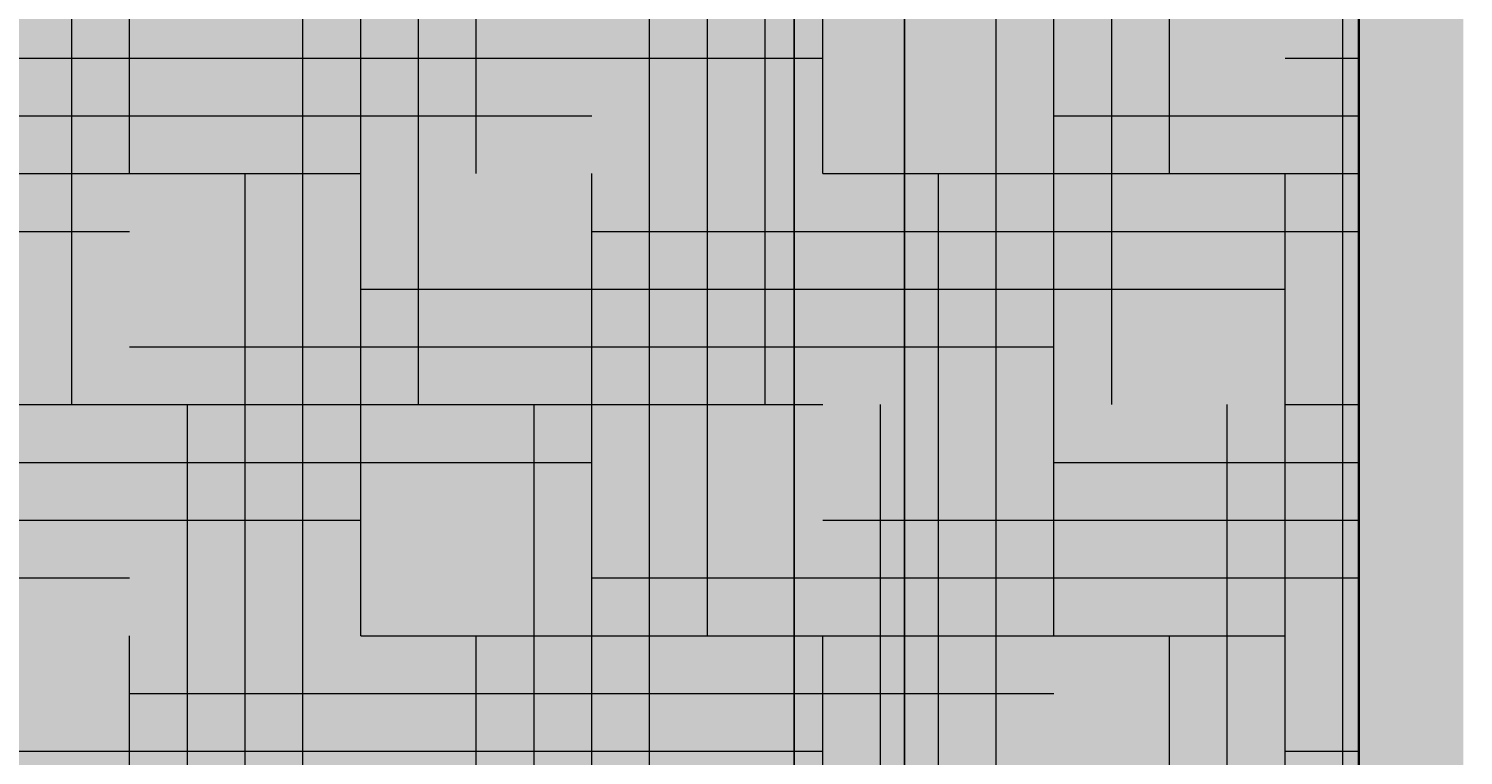
# Model space of a CAD drawing. Units: feet. Extents: x 2695 to 2912, y 795 to 1139.
# Tile 8 of 83: x 2734 to 2774, y 835 to 855. Entities that reach past the tile are written whole.
import ezdxf

# ---------------------------------------------------------------- set-up
doc = ezdxf.new("R2010")
doc.units = ezdxf.units.FT
for name, color, linetype, lineweight in [('A-ANNO-DIMS', 2, 'Continuous', 18), ('A-ELEV', 7, 'Continuous', 35), ('A-ELEV-PATT', 252, 'Continuous', 13)]:
    doc.layers.add(name, color=color, linetype=linetype, lineweight=lineweight)
doc.styles.get("Standard").update_dxf_attribs({"font": 'arial.ttf'})
doc.dimstyles.get("Standard").update_dxf_attribs({"dimtxt": 0.18, "dimasz": 0.18, "dimexe": 0.18, "dimexo": 0.0625, "dimgap": 0.09, "dimtad": 0, "dimtih": 1, "dimtoh": 1, "dimdec": 1, "dimzin": 0, "dimdsep": 46, "dimlunit": 3, "dimtxsty": 'Standard', "dimcen": 0.09, "dimadec": 0, "dimazin": 0, "dimtfac": 1, "dimtdec": 1, "dimtofl": 0, "dimtmove": 0, "dimatfit": 3, "dimfxl": 1, "dimtolj": 1, "dimtzin": 0, "dimarcsym": 0})

# ---------------------------------------------------------------- blocks, each defined once
blk = doc.blocks.new('*D3')
at = {"layer": 'A-ANNO-DIMS', "color": 0, "lineweight": -2, "transparency": 16777216}
for p, q in [((2724.189, 874.795), (2724.189, 794.976)), ((2758.151, 874.795), (2758.151, 794.976)), ((2724.369, 795.156), (2740.777, 795.156)), ((2757.971, 795.156), (2741.564, 795.156))]:
    blk.add_line(p, q, dxfattribs=at)
at = {"layer": 'A-ANNO-DIMS', "color": 0, "transparency": 16777216}
for points in [[(2724.369, 795.186), (2724.369, 795.126), (2724.189, 795.156)], [(2757.971, 795.186), (2757.971, 795.126), (2758.151, 795.156)]]:
    blk.add_solid(points, dxfattribs=at)
at = {"layer": 'Defpoints', "color": 0, "transparency": 16777216}
for p in [(2724.189, 874.857), (2758.151, 874.857), (2758.151, 795.156)]:
    blk.add_point(p, dxfattribs=at)
at = {"layer": 'A-ANNO-DIMS', "color": 0, "transparency": 16777216, "insert": (2741.17, 795.156), "char_height": 0.18, "attachment_point": 5}
blk.add_mtext('\\A1;33.96', dxfattribs=at)
blk = doc.blocks.new('*D4')
at = {"layer": 'A-ANNO-DIMS', "color": 0, "lineweight": -2, "transparency": 16777216}
for p, q in [((2758.151, 874.795), (2758.151, 794.976)), ((2773.503, 810.868), (2773.503, 794.976)), ((2758.331, 795.156), (2765.441, 795.156)), ((2773.323, 795.156), (2766.213, 795.156))]:
    blk.add_line(p, q, dxfattribs=at)
at = {"layer": 'A-ANNO-DIMS', "color": 0, "transparency": 16777216}
for points in [[(2758.331, 795.186), (2758.331, 795.126), (2758.151, 795.156)], [(2773.323, 795.186), (2773.323, 795.126), (2773.503, 795.156)]]:
    blk.add_solid(points, dxfattribs=at)
at = {"layer": 'Defpoints', "color": 0, "transparency": 16777216}
for p in [(2758.151, 874.857), (2773.503, 810.931), (2773.503, 795.156)]:
    blk.add_point(p, dxfattribs=at)
at = {"layer": 'A-ANNO-DIMS', "color": 0, "transparency": 16777216, "insert": (2765.827, 795.156), "char_height": 0.18, "attachment_point": 5}
blk.add_mtext('\\A1;15.35', dxfattribs=at)
blk = doc.blocks.new('*D13')
at = {"layer": 'A-ANNO-DIMS', "color": 0, "lineweight": -2, "transparency": 16777216}
for p, q in [((2758.214, 874.857), (2911.424, 874.857)), ((2911.244, 874.677), (2911.244, 843.076)), ((2911.244, 811.111), (2911.244, 842.712)), ((2890.699, 810.931), (2911.424, 810.931))]:
    blk.add_line(p, q, dxfattribs=at)
at = {"layer": 'A-ANNO-DIMS', "color": 0, "transparency": 16777216}
for points in [[(2911.214, 874.677), (2911.274, 874.677), (2911.244, 874.857)], [(2911.214, 811.111), (2911.274, 811.111), (2911.244, 810.931)]]:
    blk.add_solid(points, dxfattribs=at)
at = {"layer": 'Defpoints', "color": 0, "transparency": 16777216}
for p in [(2758.151, 874.857), (2911.244, 874.857), (2890.636, 810.931)]:
    blk.add_point(p, dxfattribs=at)
at = {"layer": 'A-ANNO-DIMS', "color": 0, "transparency": 16777216, "insert": (2911.244, 842.894), "char_height": 0.18, "attachment_point": 5}
blk.add_mtext('\\A1;63.93', dxfattribs=at)
blk = doc.blocks.new('*D24')
at = {"layer": 'A-ANNO-DIMS', "color": 0, "lineweight": -2, "transparency": 16777216}
for p, q in [((2730.708, 936.868), (2730.708, 794.976)), ((2755.112, 936.868), (2755.112, 794.976)), ((2730.888, 795.156), (2742.446, 795.156)), ((2754.932, 795.156), (2743.375, 795.156))]:
    blk.add_line(p, q, dxfattribs=at)
at = {"layer": 'A-ANNO-DIMS', "color": 0, "transparency": 16777216}
for points in [[(2730.888, 795.186), (2730.888, 795.126), (2730.708, 795.156)], [(2754.932, 795.186), (2754.932, 795.126), (2755.112, 795.156)]]:
    blk.add_solid(points, dxfattribs=at)
at = {"layer": 'Defpoints', "color": 0, "transparency": 16777216}
for p in [(2730.708, 936.931), (2755.112, 936.931), (2755.112, 795.156)]:
    blk.add_point(p, dxfattribs=at)
at = {"layer": 'A-ANNO-DIMS', "color": 0, "transparency": 16777216, "insert": (2742.91, 795.156), "char_height": 0.18, "attachment_point": 5}
blk.add_mtext('\\A1;24.404', dxfattribs=at)
blk = doc.blocks.new('*D25')
at = {"layer": 'A-ANNO-DIMS', "color": 0, "lineweight": -2, "transparency": 16777216}
for p, q in [((2755.112, 936.868), (2755.112, 794.976)), ((2770.636, 936.868), (2770.636, 794.976)), ((2755.292, 795.156), (2762.419, 795.156)), ((2770.456, 795.156), (2763.329, 795.156))]:
    blk.add_line(p, q, dxfattribs=at)
at = {"layer": 'A-ANNO-DIMS', "color": 0, "transparency": 16777216}
for points in [[(2755.292, 795.186), (2755.292, 795.126), (2755.112, 795.156)], [(2770.456, 795.186), (2770.456, 795.126), (2770.636, 795.156)]]:
    blk.add_solid(points, dxfattribs=at)
at = {"layer": 'Defpoints', "color": 0, "transparency": 16777216}
for p in [(2755.112, 936.931), (2770.636, 936.931), (2770.636, 795.156)]:
    blk.add_point(p, dxfattribs=at)
at = {"layer": 'A-ANNO-DIMS', "color": 0, "transparency": 16777216, "insert": (2762.874, 795.156), "char_height": 0.18, "attachment_point": 5}
blk.add_mtext('\\A1;15.524', dxfattribs=at)

msp = doc.modelspace()

# ---------------------------------------------------------------- hatches: boundary and pattern name
at = {"layer": 'A-ELEV-PATT'}
h = msp.add_hatch(color=256, dxfattribs=at)
h.set_gradient(color1=(147, 149, 152), color2=(147, 149, 152), tint=1)
h.paths.add_polyline_path([(2770.6361, 1118.4096), (2710.6361, 1118.4096), (2710.6361, 1062.9306), (2770.6361, 1062.9306)])
h.paths.add_polyline_path([(2890.6361, 1103.3378), (2770.6361, 1103.3378), (2770.6361, 1062.9306), (2890.6361, 1062.9306)])
h.paths.add_polyline_path([(2730.7081, 1048.1052), (2755.1125, 1048.1052), (2755.1125, 936.9306), (2770.6361, 936.9306), (2770.6361, 1050.3105), (2715.8852, 1050.3105), (2715.8852, 936.9306), (2730.7081, 936.9306)])
h.paths.add_polyline_path([(2890.6361, 1050.3105), (2770.6361, 1050.3105), (2770.6361, 971.9673), (2778.0341, 971.9673), (2778.0341, 1020.8235), (2843.575, 1020.8235), (2843.575, 971.9673), (2890.6361, 971.9673)])
h.paths.add_polyline_path([(2888.1882, 970.7156), (2843.575, 970.7156), (2843.575, 964.8267), (2888.1882, 964.8267)])
h.paths.add_polyline_path([(2888.1882, 964.1328), (2843.575, 964.1328), (2843.575, 956.614), (2888.1882, 956.614)])
h.paths.add_polyline_path([(2888.1882, 955.9202), (2843.575, 955.9202), (2843.575, 949.2892), (2888.1882, 949.2892)])
h.paths.add_polyline_path([(2888.1882, 948.5954), (2843.575, 948.5954), (2843.575, 941.3507), (2888.1882, 941.3507)])
h.paths.add_polyline_path([(2888.1882, 940.6569), (2843.575, 940.6569), (2843.575, 936.9306), (2888.1882, 936.9306)])
h.paths.add_polyline_path([(2890.6361, 970.7156), (2888.9368, 970.7156), (2888.9368, 964.8267), (2890.6361, 964.8267)])
h.paths.add_polyline_path([(2890.6361, 964.1328), (2888.9368, 964.1328), (2888.9368, 956.614), (2890.6361, 956.614)])
h.paths.add_polyline_path([(2890.6361, 955.9202), (2888.9368, 955.9202), (2888.9368, 949.2892), (2890.6361, 949.2892)])
h.paths.add_polyline_path([(2890.6361, 940.6569), (2888.9368, 940.6569), (2888.9368, 936.9306), (2890.6361, 936.9306)])
h.paths.add_polyline_path([(2890.6361, 948.5954), (2888.9368, 948.5954), (2888.9368, 941.3507), (2890.6361, 941.3507)])
h.paths.add_polyline_path([(2772.5216, 970.7156), (2770.6361, 970.7156), (2770.6361, 964.8267), (2772.5216, 964.8267)])
h.paths.add_polyline_path([(2772.5216, 964.1328), (2770.6361, 964.1328), (2770.6361, 956.614), (2772.5216, 956.614)])
h.paths.add_polyline_path([(2772.5216, 955.9202), (2770.6361, 955.9202), (2770.6361, 949.2892), (2772.5216, 949.2892)])
h.paths.add_polyline_path([(2772.5216, 948.5954), (2770.6361, 948.5954), (2770.6361, 941.3507), (2772.5216, 941.3507)])
h.paths.add_polyline_path([(2772.5216, 940.6569), (2770.6361, 940.6569), (2770.6361, 936.9306), (2772.5216, 936.9306)])
h.paths.add_polyline_path([(2778.0341, 940.6569), (2773.2702, 940.6569), (2773.2702, 936.9306), (2778.0341, 936.9306)])
h.paths.add_polyline_path([(2778.0341, 970.7156), (2773.2702, 970.7156), (2773.2702, 964.8267), (2778.0341, 964.8267)])
h.paths.add_polyline_path([(2778.0341, 964.1328), (2773.2702, 964.1328), (2773.2702, 956.614), (2778.0341, 956.614)])
h.paths.add_polyline_path([(2778.0341, 955.9202), (2773.2702, 955.9202), (2773.2702, 949.2892), (2778.0341, 949.2892)])
h.paths.add_polyline_path([(2778.0341, 948.5954), (2773.2702, 948.5954), (2773.2702, 941.3507), (2778.0341, 941.3507)])
h.paths.add_polyline_path([(2810.0407, 940.6569), (2780.0341, 940.6569), (2780.0341, 936.9306), (2810.0407, 936.9306)])
h.paths.add_polyline_path([(2890.6361, 924.3105), (2770.6361, 924.3105), (2770.6361, 810.9306), (2773.5029, 810.9306), (2773.5029, 905.5143), (2805.9398, 905.5143), (2838.3767, 905.5143), (2838.3767, 810.9306), (2890.6361, 810.9306)])
h = msp.add_hatch(color=256, dxfattribs=at)
h.set_gradient(color1=(255, 255, 255))
h.paths.add_polyline_path([(2770.6361, 924.3105), (2716.5358, 924.3105), (2716.5358, 810.9306), (2770.6361, 810.9306)])
h.paths.add_polyline_path([(2758.1515, 902.577), (2758.1515, 874.8571), (2724.1893, 874.8571), (2724.1893, 902.577)], flags=16)
h.paths.add_polyline_path([(2756.1515, 900.577), (2756.1515, 876.8571), (2726.1893, 876.8571), (2726.1893, 900.577)], flags=0)
h.paths.add_polyline_path([(2740.7302, 900.577), (2741.6105, 900.577), (2741.6105, 876.8571), (2740.7302, 876.8571)], flags=0)
h = msp.add_hatch(dxfattribs=at)
h.set_pattern_fill('HOUND', color=256, style=0)
h.paths.add_polyline_path([(2770.6361, 924.3105), (2716.5358, 924.3105), (2716.5358, 810.9306), (2770.6361, 810.9306)])
h.paths.add_polyline_path([(2724.1893, 874.8571), (2724.1893, 902.577), (2758.1515, 902.577), (2758.1515, 874.8571)], flags=16)
h.paths.add_polyline_path([(2756.1515, 876.8571), (2726.1893, 876.8571), (2726.1893, 900.577), (2756.1515, 900.577)], flags=0)
h.paths.add_polyline_path([(2741.6105, 876.8571), (2740.7302, 876.8571), (2740.7302, 900.577), (2741.6105, 900.577)], flags=0)

# ---------------------------------------------------------------- linework, layer by layer
at = {"layer": 'A-ELEV'}
for p, q in [((2770.6361, 924.3105), (2770.6361, 810.9306)), ((2770.6361, 810.9306), (2770.6361, 924.3105))]:
    msp.add_line(p, q, dxfattribs=at)
msp.add_lwpolyline([(2716.5358, 924.3105), (2770.6361, 924.3105), (2770.6361, 810.9306), (2716.5358, 810.9306)], close=True, dxfattribs=at)

# ---------------------------------------------------------------- dimensions: what is measured, and where the dimension line sits
at = {"layer": 'A-ANNO-DIMS'}
for base, p1, p2, override, picture, middle in [((2755.1125, 795.1556), (2730.7081, 936.9306), (2755.1125, 936.9306), {"dimdec": 3, "dimlfac": 1, "dimrnd": 0, "dimzin": 0, "dimdsep": 46, "dimlunit": 2}, '*D24', (2742.9103, 795.1556)), ((2770.6361, 795.1556), (2755.1125, 936.9306), (2770.6361, 936.9306), {"dimdec": 3, "dimlfac": 1, "dimrnd": 0, "dimzin": 0, "dimdsep": 46, "dimlunit": 2}, '*D25', (2762.8743, 795.1556)), ((2758.1515, 795.1556), (2724.1893, 874.8571), (2758.1515, 874.8571), {"dimdec": 2, "dimlfac": 1, "dimrnd": 0, "dimzin": 0, "dimdsep": 46, "dimlunit": 2}, '*D3', (2741.1704, 795.1556)), ((2773.5029, 795.1556), (2758.1515, 874.8571), (2773.5029, 810.9306), {"dimdec": 2, "dimlfac": 1, "dimrnd": 0, "dimzin": 0, "dimdsep": 46, "dimlunit": 2}, '*D4', (2765.8272, 795.1556))]:
    dim = msp.add_linear_dim(base=base, p1=p1, p2=p2, dimstyle='Standard', override=override, dxfattribs=at)
    dim.commit()
    dim.dimension.update_dxf_attribs({"geometry": picture, "text_midpoint": middle})
dim = msp.add_linear_dim(base=(2911.2444, 874.8571), p1=(2890.6361, 810.9306), p2=(2758.1515, 874.8571), angle=90, dimstyle='Standard', override={"dimdec": 2, "dimlfac": 1, "dimrnd": 0, "dimzin": 0, "dimdsep": 46, "dimlunit": 2}, dxfattribs=at)
dim.commit()
dim.dimension.update_dxf_attribs({"geometry": '*D13', "text_midpoint": (2911.2444, 842.8938)})

doc.saveas('drawing.dxf')
